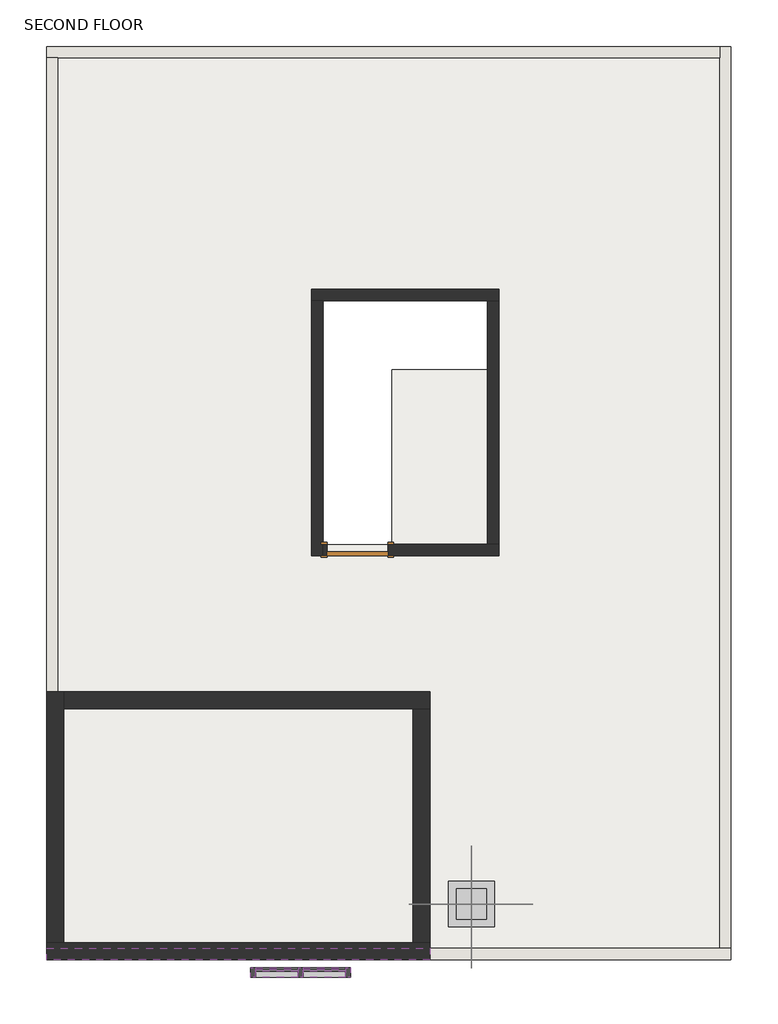
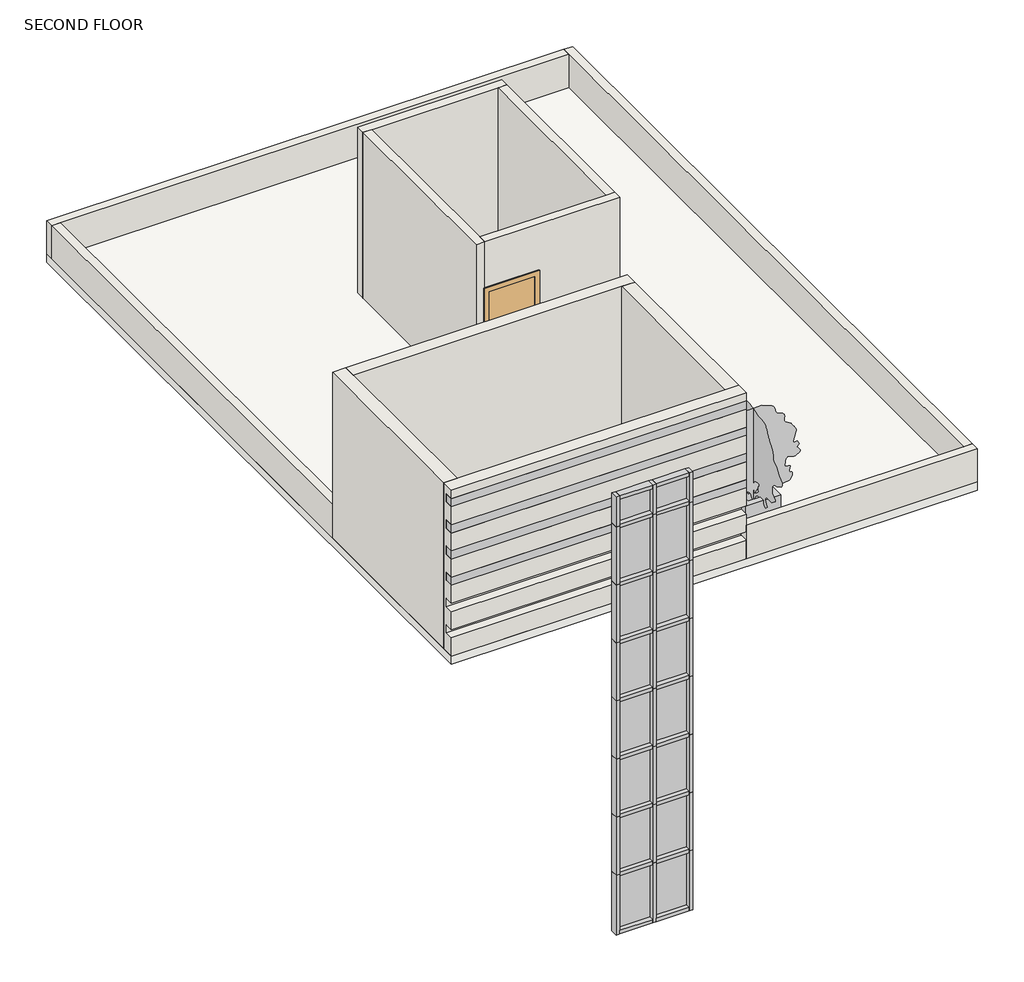
# One storey, incomplete: 42 members, 16 plates, 12 walls, 4 proxies, 2 geographic elements, 1 door, 1 slab.
"""IFC4 building model written with IfcOpenShell, lengths in millimetres."""

from ifc_helpers import new_model, si_unit, frame, origin, place, context, project, spatial, polyline, outline, extrude, faceted_brep, transform, mapped, element, save
from components import door_377e7377, planter_2_x2_da431093, rpc_tree_deciduous_largetooth_aspen_25_807f66b4, member_e80433b6, member_69c8e218, member_c8189573, member_de12db52, member_a715cb85, member_3683b620, member_544ec0ca, member_c4de40ee, system_panel_glazed_b36dd56d, system_panel_glazed_61a83ab7

model = new_model("IFC4")

# Units and contexts
model_context = context("Model", 3, world=origin())
ifc_project = project(units=[si_unit("LENGTHUNIT", "METRE", prefix="MILLI")], contexts=[model_context])

# Site, building, storey
site = spatial("IfcSite", under=ifc_project)
building = spatial("IfcBuilding", under=site)
storey = spatial("IfcBuildingStorey", under=building, Name="SECOND FLOOR", Elevation=6400.8)

# Proxies
placement = place(None, origin())
element("IfcBuildingElementProxy", 1, Name="Reveal", ObjectType="Reveal", at=placement, inside=storey, context=model_context, shape_type="SweptSolid", body=[
    extrude(outline(polyline([(-5827.2415084, -5557.8064015), (-5827.2415084, -5405.4064015), (-702.7915084, -5405.4064015), (-702.7915084, -5557.8064015), (-5827.2415084, -5557.8064015)])), frame((0.0, 0.0, 9144.0), z_axis=(0.0, 0.0, 1.0), x_axis=(1.0, 0.0, 0.0)), (0.0, 0.0, 1.0), 152.4),
])
element("IfcBuildingElementProxy", 2, Name="Reveal", ObjectType="Reveal", at=placement, inside=storey, context=model_context, shape_type="SweptSolid", body=[
    extrude(outline(polyline([(-5827.2415084, -5557.8064015), (-5827.2415084, -5405.4064015), (-702.7915084, -5405.4064015), (-702.7915084, -5557.8064015), (-5827.2415084, -5557.8064015)])), frame((0.0, 0.0, 8662.7368421), z_axis=(0.0, 0.0, 1.0), x_axis=(1.0, 0.0, 0.0)), (0.0, 0.0, 1.0), 152.4),
])
element("IfcBuildingElementProxy", 3, Name="Reveal", ObjectType="Reveal", at=placement, inside=storey, context=model_context, shape_type="SweptSolid", body=[
    extrude(outline(polyline([(-5827.2415084, -5557.8064015), (-5827.2415084, -5405.4064015), (-702.7915084, -5405.4064015), (-702.7915084, -5557.8064015), (-5827.2415084, -5557.8064015)])), frame((0.0, 0.0, 8181.4736842), z_axis=(0.0, 0.0, 1.0), x_axis=(1.0, 0.0, 0.0)), (0.0, 0.0, 1.0), 152.4),
])
element("IfcBuildingElementProxy", 4, Name="Reveal", ObjectType="Reveal", at=placement, inside=storey, context=model_context, shape_type="SweptSolid", body=[
    extrude(outline(polyline([(-5827.2415084, -5557.8064015), (-5827.2415084, -5405.4064015), (-702.7915084, -5405.4064015), (-702.7915084, -5557.8064015), (-5827.2415084, -5557.8064015)])), frame((0.0, 0.0, 7700.2105263), z_axis=(0.0, 0.0, 1.0), x_axis=(1.0, 0.0, 0.0)), (0.0, 0.0, 1.0), 152.4),
])

# Door
door_shape = door_377e7377(model_context)
element("IfcDoor", 5, ObjectType="Single-Flush : 2'8\"X7'", at=placement, inside=storey, context=model_context, shape_type="MappedRepresentation", body=[
    mapped(door_shape, transform((-1674.3415084, -85.6533727, 6400.8), x_axis=(-1.0, 0.0, 0.0), y_axis=(0.0, -1.0, 0.0), z_axis=(0.0, 0.0, 1.0))),
])

# Geographic elements
planter_2_x2_shape = planter_2_x2_da431093(model_context)
element("IfcGeographicElement", 6, ObjectType="Planter : 2'x2'", at=placement, inside=storey, context=model_context, shape_type="MappedRepresentation", body=[
    mapped(planter_2_x2_shape, transform((-150.3415084, -4814.8564015, 6400.8), x_axis=(1.0, 0.0, 0.0), y_axis=(0.0, 1.0, 0.0), z_axis=(0.0, 0.0, 1.0))),
])
rpc_tree_deciduous_largetooth_aspen_25_shape = rpc_tree_deciduous_largetooth_aspen_25_807f66b4(model_context)
element("IfcGeographicElement", 7, ObjectType="RPC Tree - Deciduous : Largetooth Aspen - 25'", at=placement, inside=storey, context=model_context, shape_type="MappedRepresentation", body=[
    mapped(rpc_tree_deciduous_largetooth_aspen_25_shape, transform((-150.3415084, -4814.8564015, 6400.8), x_axis=(1.0, 0.0, 0.0), y_axis=(0.0, 1.0, 0.0), z_axis=(0.0, 0.0, 1.0))),
])

# Members
member_shape = member_e80433b6(model_context)
element("IfcMember", 8, ObjectType="Rectangular Mullion : 2.5\" x 5\" rectangular", at=placement, inside=storey, context=model_context, shape_type="MappedRepresentation", body=[
    mapped(member_shape, transform((-2433.3720223, -5729.2564015, 462.2131579), x_axis=(1.0, 0.0, 0.0), y_axis=(0.0, -1.0, 0.0), z_axis=(0.0, 0.0, -1.0))),
])
member_2_shape = member_69c8e218(model_context)
element("IfcMember", 9, ObjectType="Rectangular Mullion : 2.5\" x 5\" rectangular", at=placement, inside=storey, context=model_context, shape_type="MappedRepresentation", body=[
    mapped(member_2_shape, transform((-1766.6220223, -5729.2564015, 462.2131579), x_axis=(1.0, 0.0, 0.0), y_axis=(0.0, -1.0, 0.0), z_axis=(0.0, 0.0, -1.0))),
])
member_3_shape = member_c8189573(model_context)
element("IfcMember", 10, ObjectType="Rectangular Mullion : 2.5\" x 5\" rectangular", at=placement, inside=storey, context=model_context, shape_type="MappedRepresentation", body=[
    mapped(member_3_shape, transform((-1830.1220223, -5729.2564015, 8510.3368421), x_axis=(0.0, 0.0, 1.0), y_axis=(0.0, -1.0, 0.0), z_axis=(1.0, 0.0, 0.0))),
])
element("IfcMember", 11, ObjectType="Rectangular Mullion : 2.5\" x 5\" rectangular", at=placement, inside=storey, context=model_context, shape_type="MappedRepresentation", body=[
    mapped(member_3_shape, transform((-2465.1220223, -5729.2564015, 8510.3368421), x_axis=(0.0, 0.0, 1.0), y_axis=(0.0, -1.0, 0.0), z_axis=(1.0, 0.0, 0.0))),
])
element("IfcMember", 12, ObjectType="Rectangular Mullion : 2.5\" x 5\" rectangular", at=placement, inside=storey, context=model_context, shape_type="MappedRepresentation", body=[
    mapped(member_3_shape, transform((-3036.6220223, -5729.2564015, 462.2131579), x_axis=(0.0, 0.0, -1.0), y_axis=(0.0, -1.0, 0.0), z_axis=(-1.0, 0.0, 0.0))),
])
element("IfcMember", 13, ObjectType="Rectangular Mullion : 2.5\" x 5\" rectangular", at=placement, inside=storey, context=model_context, shape_type="MappedRepresentation", body=[
    mapped(member_3_shape, transform((-2401.6220223, -5729.2564015, 462.2131579), x_axis=(0.0, 0.0, -1.0), y_axis=(0.0, -1.0, 0.0), z_axis=(-1.0, 0.0, 0.0))),
])
member_4_shape = member_de12db52(model_context)
element("IfcMember", 14, ObjectType="Rectangular Mullion : 2.5\" x 5\" rectangular", at=placement, inside=storey, context=model_context, shape_type="MappedRepresentation", body=[
    mapped(member_4_shape, transform((-2465.1220223, -5729.2564015, 1560.7631579), x_axis=(0.0, 0.0, 1.0), y_axis=(0.0, -1.0, 0.0), z_axis=(1.0, 0.0, 0.0))),
])
element("IfcMember", 15, ObjectType="Rectangular Mullion : 2.5\" x 5\" rectangular", at=placement, inside=storey, context=model_context, shape_type="MappedRepresentation", body=[
    mapped(member_4_shape, transform((-2465.1220223, -5729.2564015, 2627.5631579), x_axis=(0.0, 0.0, 1.0), y_axis=(0.0, -1.0, 0.0), z_axis=(1.0, 0.0, 0.0))),
])
element("IfcMember", 16, ObjectType="Rectangular Mullion : 2.5\" x 5\" rectangular", at=placement, inside=storey, context=model_context, shape_type="MappedRepresentation", body=[
    mapped(member_4_shape, transform((-2465.1220223, -5729.2564015, 3694.3631579), x_axis=(0.0, 0.0, 1.0), y_axis=(0.0, -1.0, 0.0), z_axis=(1.0, 0.0, 0.0))),
])
element("IfcMember", 17, ObjectType="Rectangular Mullion : 2.5\" x 5\" rectangular", at=placement, inside=storey, context=model_context, shape_type="MappedRepresentation", body=[
    mapped(member_4_shape, transform((-1830.1220223, -5729.2564015, 1560.7631579), x_axis=(0.0, 0.0, 1.0), y_axis=(0.0, -1.0, 0.0), z_axis=(1.0, 0.0, 0.0))),
])
element("IfcMember", 18, ObjectType="Rectangular Mullion : 2.5\" x 5\" rectangular", at=placement, inside=storey, context=model_context, shape_type="MappedRepresentation", body=[
    mapped(member_4_shape, transform((-1830.1220223, -5729.2564015, 2627.5631579), x_axis=(0.0, 0.0, 1.0), y_axis=(0.0, -1.0, 0.0), z_axis=(1.0, 0.0, 0.0))),
])
element("IfcMember", 19, ObjectType="Rectangular Mullion : 2.5\" x 5\" rectangular", at=placement, inside=storey, context=model_context, shape_type="MappedRepresentation", body=[
    mapped(member_4_shape, transform((-1830.1220223, -5729.2564015, 3694.3631579), x_axis=(0.0, 0.0, 1.0), y_axis=(0.0, -1.0, 0.0), z_axis=(1.0, 0.0, 0.0))),
])
element("IfcMember", 20, ObjectType="Rectangular Mullion : 2.5\" x 5\" rectangular", at=placement, inside=storey, context=model_context, shape_type="MappedRepresentation", body=[
    mapped(member_4_shape, transform((-2465.1220223, -5729.2564015, 4761.1631579), x_axis=(0.0, 0.0, 1.0), y_axis=(0.0, -1.0, 0.0), z_axis=(1.0, 0.0, 0.0))),
])
element("IfcMember", 21, ObjectType="Rectangular Mullion : 2.5\" x 5\" rectangular", at=placement, inside=storey, context=model_context, shape_type="MappedRepresentation", body=[
    mapped(member_4_shape, transform((-1830.1220223, -5729.2564015, 4761.1631579), x_axis=(0.0, 0.0, 1.0), y_axis=(0.0, -1.0, 0.0), z_axis=(1.0, 0.0, 0.0))),
])
element("IfcMember", 22, ObjectType="Rectangular Mullion : 2.5\" x 5\" rectangular", at=placement, inside=storey, context=model_context, shape_type="MappedRepresentation", body=[
    mapped(member_4_shape, transform((-2465.1220223, -5729.2564015, 5827.9631579), x_axis=(0.0, 0.0, 1.0), y_axis=(0.0, -1.0, 0.0), z_axis=(1.0, 0.0, 0.0))),
])
element("IfcMember", 23, ObjectType="Rectangular Mullion : 2.5\" x 5\" rectangular", at=placement, inside=storey, context=model_context, shape_type="MappedRepresentation", body=[
    mapped(member_4_shape, transform((-1830.1220223, -5729.2564015, 5827.9631579), x_axis=(0.0, 0.0, 1.0), y_axis=(0.0, -1.0, 0.0), z_axis=(1.0, 0.0, 0.0))),
])
element("IfcMember", 24, ObjectType="Rectangular Mullion : 2.5\" x 5\" rectangular", at=placement, inside=storey, context=model_context, shape_type="MappedRepresentation", body=[
    mapped(member_4_shape, transform((-2465.1220223, -5729.2564015, 6894.7631579), x_axis=(0.0, 0.0, 1.0), y_axis=(0.0, -1.0, 0.0), z_axis=(1.0, 0.0, 0.0))),
])
element("IfcMember", 25, ObjectType="Rectangular Mullion : 2.5\" x 5\" rectangular", at=placement, inside=storey, context=model_context, shape_type="MappedRepresentation", body=[
    mapped(member_4_shape, transform((-1830.1220223, -5729.2564015, 6894.7631579), x_axis=(0.0, 0.0, 1.0), y_axis=(0.0, -1.0, 0.0), z_axis=(1.0, 0.0, 0.0))),
])
element("IfcMember", 26, ObjectType="Rectangular Mullion : 2.5\" x 5\" rectangular", at=placement, inside=storey, context=model_context, shape_type="MappedRepresentation", body=[
    mapped(member_4_shape, transform((-2465.1220223, -5729.2564015, 7961.5631579), x_axis=(0.0, 0.0, 1.0), y_axis=(0.0, -1.0, 0.0), z_axis=(1.0, 0.0, 0.0))),
])
element("IfcMember", 27, ObjectType="Rectangular Mullion : 2.5\" x 5\" rectangular", at=placement, inside=storey, context=model_context, shape_type="MappedRepresentation", body=[
    mapped(member_4_shape, transform((-1830.1220223, -5729.2564015, 7961.5631579), x_axis=(0.0, 0.0, 1.0), y_axis=(0.0, -1.0, 0.0), z_axis=(1.0, 0.0, 0.0))),
])
member_5_shape = member_a715cb85(model_context)
element("IfcMember", 28, ObjectType="Rectangular Mullion : 2.5\" x 5\" rectangular", at=placement, inside=storey, context=model_context, shape_type="MappedRepresentation", body=[
    mapped(member_5_shape, transform((-2433.3720223, -5729.2564015, 1560.7631579), x_axis=(1.0, 0.0, 0.0), y_axis=(0.0, -1.0, 0.0), z_axis=(0.0, 0.0, -1.0))),
])
element("IfcMember", 29, ObjectType="Rectangular Mullion : 2.5\" x 5\" rectangular", at=placement, inside=storey, context=model_context, shape_type="MappedRepresentation", body=[
    mapped(member_5_shape, transform((-2433.3720223, -5729.2564015, 2627.5631579), x_axis=(1.0, 0.0, 0.0), y_axis=(0.0, -1.0, 0.0), z_axis=(0.0, 0.0, -1.0))),
])
element("IfcMember", 30, ObjectType="Rectangular Mullion : 2.5\" x 5\" rectangular", at=placement, inside=storey, context=model_context, shape_type="MappedRepresentation", body=[
    mapped(member_5_shape, transform((-2433.3720223, -5729.2564015, 3694.3631579), x_axis=(1.0, 0.0, 0.0), y_axis=(0.0, -1.0, 0.0), z_axis=(0.0, 0.0, -1.0))),
])
element("IfcMember", 31, ObjectType="Rectangular Mullion : 2.5\" x 5\" rectangular", at=placement, inside=storey, context=model_context, shape_type="MappedRepresentation", body=[
    mapped(member_5_shape, transform((-2433.3720223, -5729.2564015, 4761.1631579), x_axis=(1.0, 0.0, 0.0), y_axis=(0.0, -1.0, 0.0), z_axis=(0.0, 0.0, -1.0))),
])
element("IfcMember", 32, ObjectType="Rectangular Mullion : 2.5\" x 5\" rectangular", at=placement, inside=storey, context=model_context, shape_type="MappedRepresentation", body=[
    mapped(member_5_shape, transform((-2433.3720223, -5729.2564015, 5827.9631579), x_axis=(1.0, 0.0, 0.0), y_axis=(0.0, -1.0, 0.0), z_axis=(0.0, 0.0, -1.0))),
])
element("IfcMember", 33, ObjectType="Rectangular Mullion : 2.5\" x 5\" rectangular", at=placement, inside=storey, context=model_context, shape_type="MappedRepresentation", body=[
    mapped(member_5_shape, transform((-2433.3720223, -5729.2564015, 6894.7631579), x_axis=(1.0, 0.0, 0.0), y_axis=(0.0, -1.0, 0.0), z_axis=(0.0, 0.0, -1.0))),
])
member_6_shape = member_3683b620(model_context)
element("IfcMember", 34, ObjectType="Rectangular Mullion : 2.5\" x 5\" rectangular", at=placement, inside=storey, context=model_context, shape_type="MappedRepresentation", body=[
    mapped(member_6_shape, transform((-2433.3720223, -5729.2564015, 7961.5631579), x_axis=(1.0, 0.0, 0.0), y_axis=(0.0, -1.0, 0.0), z_axis=(0.0, 0.0, -1.0))),
])
member_7_shape = member_544ec0ca(model_context)
element("IfcMember", 35, ObjectType="Rectangular Mullion : 2.5\" x 5\" rectangular", at=placement, inside=storey, context=model_context, shape_type="MappedRepresentation", body=[
    mapped(member_7_shape, transform((-3100.1220223, -5729.2564015, 8510.3368421), x_axis=(-1.0, 0.0, 0.0), y_axis=(0.0, -1.0, 0.0), z_axis=(0.0, 0.0, 1.0))),
])
member_8_shape = member_c4de40ee(model_context)
element("IfcMember", 36, ObjectType="Rectangular Mullion : 2.5\" x 5\" rectangular", at=placement, inside=storey, context=model_context, shape_type="MappedRepresentation", body=[
    mapped(member_8_shape, transform((-1766.6220223, -5729.2564015, 1560.7631579), x_axis=(1.0, 0.0, 0.0), y_axis=(0.0, -1.0, 0.0), z_axis=(0.0, 0.0, -1.0))),
])
element("IfcMember", 37, ObjectType="Rectangular Mullion : 2.5\" x 5\" rectangular", at=placement, inside=storey, context=model_context, shape_type="MappedRepresentation", body=[
    mapped(member_8_shape, transform((-1766.6220223, -5729.2564015, 2627.5631579), x_axis=(1.0, 0.0, 0.0), y_axis=(0.0, -1.0, 0.0), z_axis=(0.0, 0.0, -1.0))),
])
element("IfcMember", 38, ObjectType="Rectangular Mullion : 2.5\" x 5\" rectangular", at=placement, inside=storey, context=model_context, shape_type="MappedRepresentation", body=[
    mapped(member_8_shape, transform((-1766.6220223, -5729.2564015, 3694.3631579), x_axis=(1.0, 0.0, 0.0), y_axis=(0.0, -1.0, 0.0), z_axis=(0.0, 0.0, -1.0))),
])
element("IfcMember", 39, ObjectType="Rectangular Mullion : 2.5\" x 5\" rectangular", at=placement, inside=storey, context=model_context, shape_type="MappedRepresentation", body=[
    mapped(member_8_shape, transform((-1766.6220223, -5729.2564015, 4761.1631579), x_axis=(1.0, 0.0, 0.0), y_axis=(0.0, -1.0, 0.0), z_axis=(0.0, 0.0, -1.0))),
])
element("IfcMember", 40, ObjectType="Rectangular Mullion : 2.5\" x 5\" rectangular", at=placement, inside=storey, context=model_context, shape_type="MappedRepresentation", body=[
    mapped(member_8_shape, transform((-1766.6220223, -5729.2564015, 5827.9631579), x_axis=(1.0, 0.0, 0.0), y_axis=(0.0, -1.0, 0.0), z_axis=(0.0, 0.0, -1.0))),
])
element("IfcMember", 41, ObjectType="Rectangular Mullion : 2.5\" x 5\" rectangular", at=placement, inside=storey, context=model_context, shape_type="MappedRepresentation", body=[
    mapped(member_8_shape, transform((-1766.6220223, -5729.2564015, 6894.7631579), x_axis=(1.0, 0.0, 0.0), y_axis=(0.0, -1.0, 0.0), z_axis=(0.0, 0.0, -1.0))),
])
element("IfcMember", 42, ObjectType="Rectangular Mullion : 2.5\" x 5\" rectangular", at=placement, inside=storey, context=model_context, shape_type="MappedRepresentation", body=[
    mapped(member_2_shape, transform((-3100.1220223, -5729.2564015, 1560.7631579), x_axis=(-1.0, 0.0, 0.0), y_axis=(0.0, -1.0, 0.0), z_axis=(0.0, 0.0, 1.0))),
])
element("IfcMember", 43, ObjectType="Rectangular Mullion : 2.5\" x 5\" rectangular", at=placement, inside=storey, context=model_context, shape_type="MappedRepresentation", body=[
    mapped(member_8_shape, transform((-3100.1220223, -5729.2564015, 2627.5631579), x_axis=(-1.0, 0.0, 0.0), y_axis=(0.0, -1.0, 0.0), z_axis=(0.0, 0.0, 1.0))),
])
element("IfcMember", 44, ObjectType="Rectangular Mullion : 2.5\" x 5\" rectangular", at=placement, inside=storey, context=model_context, shape_type="MappedRepresentation", body=[
    mapped(member_8_shape, transform((-3100.1220223, -5729.2564015, 3694.3631579), x_axis=(-1.0, 0.0, 0.0), y_axis=(0.0, -1.0, 0.0), z_axis=(0.0, 0.0, 1.0))),
])
element("IfcMember", 45, ObjectType="Rectangular Mullion : 2.5\" x 5\" rectangular", at=placement, inside=storey, context=model_context, shape_type="MappedRepresentation", body=[
    mapped(member_8_shape, transform((-3100.1220223, -5729.2564015, 4761.1631579), x_axis=(-1.0, 0.0, 0.0), y_axis=(0.0, -1.0, 0.0), z_axis=(0.0, 0.0, 1.0))),
])
element("IfcMember", 46, ObjectType="Rectangular Mullion : 2.5\" x 5\" rectangular", at=placement, inside=storey, context=model_context, shape_type="MappedRepresentation", body=[
    mapped(member_8_shape, transform((-3100.1220223, -5729.2564015, 5827.9631579), x_axis=(-1.0, 0.0, 0.0), y_axis=(0.0, -1.0, 0.0), z_axis=(0.0, 0.0, 1.0))),
])
element("IfcMember", 47, ObjectType="Rectangular Mullion : 2.5\" x 5\" rectangular", at=placement, inside=storey, context=model_context, shape_type="MappedRepresentation", body=[
    mapped(member_8_shape, transform((-3100.1220223, -5729.2564015, 6894.7631579), x_axis=(-1.0, 0.0, 0.0), y_axis=(0.0, -1.0, 0.0), z_axis=(0.0, 0.0, 1.0))),
])
element("IfcMember", 48, ObjectType="Rectangular Mullion : 2.5\" x 5\" rectangular", at=placement, inside=storey, context=model_context, shape_type="MappedRepresentation", body=[
    mapped(member_8_shape, transform((-3100.1220223, -5729.2564015, 7961.5631579), x_axis=(-1.0, 0.0, 0.0), y_axis=(0.0, -1.0, 0.0), z_axis=(0.0, 0.0, 1.0))),
])
element("IfcMember", 49, ObjectType="Rectangular Mullion : 2.5\" x 5\" rectangular", at=placement, inside=storey, context=model_context, shape_type="MappedRepresentation", body=[
    mapped(member_7_shape, transform((-1766.6220223, -5729.2564015, 7961.5631579), x_axis=(1.0, 0.0, 0.0), y_axis=(0.0, -1.0, 0.0), z_axis=(0.0, 0.0, -1.0))),
])

# Plates
system_panel_glazed_shape = system_panel_glazed_b36dd56d(model_context)
element("IfcPlate", 50, ObjectType="System Panel : Glazed", at=placement, inside=storey, context=model_context, shape_type="MappedRepresentation", body=[
    mapped(system_panel_glazed_shape, transform((-2750.8720223, -5729.2564015, 525.7131579), x_axis=(1.0, 0.0, 0.0), y_axis=(0.0, 1.0, 0.0), z_axis=(0.0, 0.0, 1.0))),
])
element("IfcPlate", 51, ObjectType="System Panel : Glazed", at=placement, inside=storey, context=model_context, shape_type="MappedRepresentation", body=[
    mapped(system_panel_glazed_shape, transform((-2750.8720223, -5729.2564015, 1592.5131579), x_axis=(1.0, 0.0, 0.0), y_axis=(0.0, 1.0, 0.0), z_axis=(0.0, 0.0, 1.0))),
])
element("IfcPlate", 52, ObjectType="System Panel : Glazed", at=placement, inside=storey, context=model_context, shape_type="MappedRepresentation", body=[
    mapped(system_panel_glazed_shape, transform((-2750.8720223, -5729.2564015, 2659.3131579), x_axis=(1.0, 0.0, 0.0), y_axis=(0.0, 1.0, 0.0), z_axis=(0.0, 0.0, 1.0))),
])
element("IfcPlate", 53, ObjectType="System Panel : Glazed", at=placement, inside=storey, context=model_context, shape_type="MappedRepresentation", body=[
    mapped(system_panel_glazed_shape, transform((-2750.8720223, -5729.2564015, 3726.1131579), x_axis=(1.0, 0.0, 0.0), y_axis=(0.0, 1.0, 0.0), z_axis=(0.0, 0.0, 1.0))),
])
element("IfcPlate", 54, ObjectType="System Panel : Glazed", at=placement, inside=storey, context=model_context, shape_type="MappedRepresentation", body=[
    mapped(system_panel_glazed_shape, transform((-2115.8720223, -5729.2564015, 525.7131579), x_axis=(1.0, 0.0, 0.0), y_axis=(0.0, 1.0, 0.0), z_axis=(0.0, 0.0, 1.0))),
])
element("IfcPlate", 55, ObjectType="System Panel : Glazed", at=placement, inside=storey, context=model_context, shape_type="MappedRepresentation", body=[
    mapped(system_panel_glazed_shape, transform((-2115.8720223, -5729.2564015, 1592.5131579), x_axis=(1.0, 0.0, 0.0), y_axis=(0.0, 1.0, 0.0), z_axis=(0.0, 0.0, 1.0))),
])
element("IfcPlate", 56, ObjectType="System Panel : Glazed", at=placement, inside=storey, context=model_context, shape_type="MappedRepresentation", body=[
    mapped(system_panel_glazed_shape, transform((-2115.8720223, -5729.2564015, 2659.3131579), x_axis=(1.0, 0.0, 0.0), y_axis=(0.0, 1.0, 0.0), z_axis=(0.0, 0.0, 1.0))),
])
element("IfcPlate", 57, ObjectType="System Panel : Glazed", at=placement, inside=storey, context=model_context, shape_type="MappedRepresentation", body=[
    mapped(system_panel_glazed_shape, transform((-2115.8720223, -5729.2564015, 3726.1131579), x_axis=(1.0, 0.0, 0.0), y_axis=(0.0, 1.0, 0.0), z_axis=(0.0, 0.0, 1.0))),
])
element("IfcPlate", 58, ObjectType="System Panel : Glazed", at=placement, inside=storey, context=model_context, shape_type="MappedRepresentation", body=[
    mapped(system_panel_glazed_shape, transform((-2750.8720223, -5729.2564015, 4792.9131579), x_axis=(1.0, 0.0, 0.0), y_axis=(0.0, 1.0, 0.0), z_axis=(0.0, 0.0, 1.0))),
])
element("IfcPlate", 59, ObjectType="System Panel : Glazed", at=placement, inside=storey, context=model_context, shape_type="MappedRepresentation", body=[
    mapped(system_panel_glazed_shape, transform((-2115.8720223, -5729.2564015, 4792.9131579), x_axis=(1.0, 0.0, 0.0), y_axis=(0.0, 1.0, 0.0), z_axis=(0.0, 0.0, 1.0))),
])
element("IfcPlate", 60, ObjectType="System Panel : Glazed", at=placement, inside=storey, context=model_context, shape_type="MappedRepresentation", body=[
    mapped(system_panel_glazed_shape, transform((-2750.8720223, -5729.2564015, 5859.7131579), x_axis=(1.0, 0.0, 0.0), y_axis=(0.0, 1.0, 0.0), z_axis=(0.0, 0.0, 1.0))),
])
element("IfcPlate", 61, ObjectType="System Panel : Glazed", at=placement, inside=storey, context=model_context, shape_type="MappedRepresentation", body=[
    mapped(system_panel_glazed_shape, transform((-2115.8720223, -5729.2564015, 5859.7131579), x_axis=(1.0, 0.0, 0.0), y_axis=(0.0, 1.0, 0.0), z_axis=(0.0, 0.0, 1.0))),
])
element("IfcPlate", 62, ObjectType="System Panel : Glazed", at=placement, inside=storey, context=model_context, shape_type="MappedRepresentation", body=[
    mapped(system_panel_glazed_shape, transform((-2750.8720223, -5729.2564015, 6926.5131579), x_axis=(1.0, 0.0, 0.0), y_axis=(0.0, 1.0, 0.0), z_axis=(0.0, 0.0, 1.0))),
])
element("IfcPlate", 63, ObjectType="System Panel : Glazed", at=placement, inside=storey, context=model_context, shape_type="MappedRepresentation", body=[
    mapped(system_panel_glazed_shape, transform((-2115.8720223, -5729.2564015, 6926.5131579), x_axis=(1.0, 0.0, 0.0), y_axis=(0.0, 1.0, 0.0), z_axis=(0.0, 0.0, 1.0))),
])
system_panel_glazed_2_shape = system_panel_glazed_61a83ab7(model_context)
element("IfcPlate", 64, ObjectType="System Panel : Glazed", at=placement, inside=storey, context=model_context, shape_type="MappedRepresentation", body=[
    mapped(system_panel_glazed_2_shape, transform((-2750.8720223, -5729.2564015, 7993.3131579), x_axis=(1.0, 0.0, 0.0), y_axis=(0.0, 1.0, 0.0), z_axis=(0.0, 0.0, 1.0))),
])
element("IfcPlate", 65, ObjectType="System Panel : Glazed", at=placement, inside=storey, context=model_context, shape_type="MappedRepresentation", body=[
    mapped(system_panel_glazed_2_shape, transform((-2115.8720223, -5729.2564015, 7993.3131579), x_axis=(1.0, 0.0, 0.0), y_axis=(0.0, 1.0, 0.0), z_axis=(0.0, 0.0, 1.0))),
])

# Slab
element("IfcSlab", 66, ObjectType="6\"", at=placement, inside=storey, context=model_context, shape_type="SweptSolid", body=[
    extrude(outline(polyline([(3316.7584916, 6634.1935985), (3316.7584916, -5557.8064015), (-5827.2415084, -5557.8064015), (-5827.2415084, 6634.1935985), (3316.7584916, 6634.1935985)]), holes=[polyline([(-2131.5415084, 3243.2935985), (-2131.5415084, -9.4533727), (-1217.1415084, -9.4533727), (-1217.1415084, 2328.8935985), (65.5584916, 2328.8935985), (65.5584916, 3243.2935985), (-2131.5415084, 3243.2935985)])]), frame((0.0, 0.0, 6248.4), z_axis=(0.0, 0.0, 1.0), x_axis=(1.0, 0.0, 0.0)), (0.0, 0.0, 1.0), 152.4),
])

# Walls
element("IfcWall", 67, ObjectType="6\"", at=placement, inside=storey, context=model_context, shape_type="Brep", body=[
    faceted_brep([(217.9584916, 3395.6935985, 6400.8), (-2283.9415084, 3395.6935985, 6400.8), (-2283.9415084, 3395.6935985, 9448.8), (217.9584916, 3395.6935985, 9448.8), (217.9584916, 3243.2935985, 6400.8), (217.9584916, 3243.2935985, 9448.8), (65.5584916, 3243.2935985, 9448.8), (-2131.5415084, 3243.2935985, 9448.8), (-2283.9415084, 3243.2935985, 9448.8), (-2283.9415084, 3243.2935985, 6400.8), (-2131.5415084, 3243.2935985, 6400.8), (65.5584916, 3243.2935985, 6400.8)], [[[0, 1, 2, 3]], [[4, 5, 6, 7, 8, 9, 10, 11]], [[1, 0, 4, 11, 10, 9]], [[3, 2, 8, 7, 6, 5]], [[2, 1, 9, 8]], [[0, 3, 5, 4]]]),
])
element("IfcWall", 68, ObjectType="6\"", at=placement, inside=storey, context=model_context, shape_type="Brep", body=[
    faceted_brep([(-2283.9415084, 3243.2935985, 6400.8), (-2283.9415084, -161.8533727, 6400.8), (-2283.9415084, -161.8533727, 9448.8), (-2283.9415084, 3243.2935985, 9448.8), (-2131.5415084, 3243.2935985, 6400.8), (-2131.5415084, 3243.2935985, 9448.8), (-2131.5415084, -9.4533727, 9448.8), (-2131.5415084, -161.8533727, 9448.8), (-2131.5415084, -161.8533727, 6400.8), (-2131.5415084, -9.4533727, 6400.8)], [[[0, 1, 2, 3]], [[4, 5, 6, 7, 8, 9]], [[1, 0, 4, 9, 8]], [[3, 2, 7, 6, 5]], [[0, 3, 5, 4]], [[2, 1, 8, 7]]]),
])
element("IfcWall", 69, ObjectType="6\"", at=placement, inside=storey, context=model_context, shape_type="Brep", body=[
    faceted_brep([(-2131.5415084, -161.8533727, 6400.8), (-2080.7415084, -161.8533727, 6400.8), (-2080.7415084, -161.8533727, 8534.4), (-1267.9415084, -161.8533727, 8534.4), (-1267.9415084, -161.8533727, 6400.8), (217.9584916, -161.8533727, 6400.8), (217.9584916, -161.8533727, 9448.8), (-2131.5415084, -161.8533727, 9448.8), (-2080.7415084, -9.4533727, 8534.4), (-2080.7415084, -9.4533727, 6400.8), (-2131.5415084, -9.4533727, 6400.8), (-2131.5415084, -9.4533727, 9448.8), (65.5584916, -9.4533727, 9448.8), (217.9584916, -9.4533727, 9448.8), (217.9584916, -9.4533727, 6400.8), (65.5584916, -9.4533727, 6400.8), (-1267.9415084, -9.4533727, 6400.8), (-1267.9415084, -9.4533727, 8534.4)], [[[0, 1, 2, 3, 4, 5, 6, 7]], [[8, 9, 10, 11, 12, 13, 14, 15, 16, 17]], [[10, 9, 1, 0]], [[16, 15, 14, 5, 4]], [[7, 6, 13, 12, 11]], [[0, 7, 11, 10]], [[6, 5, 14, 13]], [[2, 1, 9, 8]], [[3, 2, 8, 17]], [[4, 3, 17, 16]]]),
])
element("IfcWall", 70, ObjectType="6\"", at=placement, inside=storey, context=model_context, shape_type="SweptSolid", body=[
    extrude(outline(polyline([(217.9584916, 3243.2935985), (217.9584916, -9.4533727), (65.5584916, -9.4533727), (65.5584916, 3243.2935985), (217.9584916, 3243.2935985)])), frame((0.0, 0.0, 6400.8), z_axis=(0.0, 0.0, 1.0), x_axis=(1.0, 0.0, 0.0)), (0.0, 0.0, 1.0), 3048.0),
])
element("IfcWall", 71, ObjectType="6\"", at=placement, inside=storey, context=model_context, shape_type="Brep", body=[
    faceted_brep([(-702.7915084, -5557.8064015, 6400.8), (3316.7584916, -5557.8064015, 6400.8), (3316.7584916, -5557.8064015, 7010.4), (-702.7915084, -5557.8064015, 7010.4), (-702.7915084, -5557.8064015, 6890.0842105), (-702.7915084, -5557.8064015, 6737.6842105), (-702.7915084, -5405.4064015, 6400.8), (-702.7915084, -5405.4064015, 7010.4), (3164.3584916, -5405.4064015, 7010.4), (3316.7584916, -5405.4064015, 7010.4), (3316.7584916, -5405.4064015, 6400.8), (3164.3584916, -5405.4064015, 6400.8)], [[[0, 1, 2, 3, 4, 5]], [[6, 7, 8, 9, 10, 11]], [[1, 0, 6, 11, 10]], [[3, 2, 9, 8, 7]], [[0, 5, 4, 3, 7, 6]], [[2, 1, 10, 9]]]),
])
element("IfcWall", 72, ObjectType="6\"", at=placement, inside=storey, context=model_context, shape_type="Brep", body=[
    faceted_brep([(3316.7584916, -5405.4064015, 6400.8), (3316.7584916, 6634.1935985, 6400.8), (3316.7584916, 6634.1935985, 7010.4), (3316.7584916, -5405.4064015, 7010.4), (3164.3584916, -5405.4064015, 6400.8), (3164.3584916, -5405.4064015, 7010.4), (3164.3584916, 6481.7935985, 7010.4), (3164.3584916, 6634.1935985, 7010.4), (3164.3584916, 6634.1935985, 6400.8), (3164.3584916, 6481.7935985, 6400.8)], [[[0, 1, 2, 3]], [[4, 5, 6, 7, 8, 9]], [[1, 0, 4, 9, 8]], [[3, 2, 7, 6, 5]], [[0, 3, 5, 4]], [[2, 1, 8, 7]]]),
])
element("IfcWall", 73, ObjectType="6\"", at=placement, inside=storey, context=model_context, shape_type="Brep", body=[
    faceted_brep([(3164.3584916, 6634.1935985, 6400.8), (-5827.2415084, 6634.1935985, 6400.8), (-5827.2415084, 6634.1935985, 7010.4), (3164.3584916, 6634.1935985, 7010.4), (3164.3584916, 6481.7935985, 6400.8), (3164.3584916, 6481.7935985, 7010.4), (-5674.8415084, 6481.7935985, 7010.4), (-5827.2415084, 6481.7935985, 7010.4), (-5827.2415084, 6481.7935985, 6400.8), (-5674.8415084, 6481.7935985, 6400.8)], [[[0, 1, 2, 3]], [[4, 5, 6, 7, 8, 9]], [[1, 0, 4, 9, 8]], [[3, 2, 7, 6, 5]], [[0, 3, 5, 4]], [[2, 1, 8, 7]]]),
])
element("IfcWall", 74, ObjectType="6\"", at=placement, inside=storey, context=model_context, shape_type="SweptSolid", body=[
    extrude(outline(polyline([(-5827.2415084, -1976.4064015), (-5827.2415084, 6481.7935985), (-5674.8415084, 6481.7935985), (-5674.8415084, -1976.4064015), (-5827.2415084, -1976.4064015)])), frame((0.0, 0.0, 6400.8), z_axis=(0.0, 0.0, 1.0), x_axis=(1.0, 0.0, 0.0)), (0.0, 0.0, 1.0), 609.6),
])
element("IfcWall", 75, ObjectType="9\"", at=placement, inside=storey, context=model_context, shape_type="Brep", body=[
    faceted_brep([(-5827.2415084, -5557.8064015, 6400.8), (-702.7915084, -5557.8064015, 6400.8), (-702.7915084, -5557.8064015, 6737.6842105), (-5827.2415084, -5557.8064015, 6737.6842105), (-702.7915084, -5557.8064015, 9448.8), (-5827.2415084, -5557.8064015, 9448.8), (-5827.2415084, -5557.8064015, 9296.4), (-702.7915084, -5557.8064015, 9296.4), (-702.7915084, -5557.8064015, 9144.0), (-5827.2415084, -5557.8064015, 9144.0), (-5827.2415084, -5557.8064015, 8815.1368421), (-702.7915084, -5557.8064015, 8815.1368421), (-5827.2415084, -5557.8064015, 6890.0842105), (-702.7915084, -5557.8064015, 6890.0842105), (-702.7915084, -5557.8064015, 7218.9473684), (-5827.2415084, -5557.8064015, 7218.9473684), (-5827.2415084, -5557.8064015, 7371.3473684), (-702.7915084, -5557.8064015, 7371.3473684), (-702.7915084, -5557.8064015, 7700.2105263), (-5827.2415084, -5557.8064015, 7700.2105263), (-5827.2415084, -5557.8064015, 7852.6105263), (-702.7915084, -5557.8064015, 7852.6105263), (-702.7915084, -5557.8064015, 8181.4736842), (-5827.2415084, -5557.8064015, 8181.4736842), (-5827.2415084, -5557.8064015, 8333.8736842), (-702.7915084, -5557.8064015, 8333.8736842), (-702.7915084, -5557.8064015, 8662.7368421), (-5827.2415084, -5557.8064015, 8662.7368421), (-702.7915084, -5329.2064015, 6400.8), (-931.3915084, -5329.2064015, 6400.8), (-5598.6415084, -5329.2064015, 6400.8), (-5827.2415084, -5329.2064015, 6400.8), (-5827.2415084, -5329.2064015, 9448.8), (-5598.6415084, -5329.2064015, 9448.8), (-931.3915084, -5329.2064015, 9448.8), (-702.7915084, -5329.2064015, 9448.8), (-702.7915084, -5405.4064015, 6400.8), (-5827.2415084, -5405.4064015, 6737.6842105), (-5827.2415084, -5405.4064015, 6890.0842105), (-5827.2415084, -5405.4064015, 7218.9473684), (-5827.2415084, -5405.4064015, 7371.3473684), (-5827.2415084, -5405.4064015, 7700.2105263), (-5827.2415084, -5405.4064015, 7852.6105263), (-5827.2415084, -5405.4064015, 8181.4736842), (-5827.2415084, -5405.4064015, 8333.8736842), (-5827.2415084, -5405.4064015, 8662.7368421), (-5827.2415084, -5405.4064015, 8815.1368421), (-5827.2415084, -5405.4064015, 9144.0), (-5827.2415084, -5405.4064015, 9296.4), (-702.7915084, -5405.4064015, 9296.4), (-702.7915084, -5405.4064015, 9144.0), (-702.7915084, -5405.4064015, 6890.0842105), (-702.7915084, -5405.4064015, 6737.6842105), (-702.7915084, -5405.4064015, 7371.3473684), (-702.7915084, -5405.4064015, 7218.9473684), (-702.7915084, -5405.4064015, 7852.6105263), (-702.7915084, -5405.4064015, 7700.2105263), (-702.7915084, -5405.4064015, 8333.8736842), (-702.7915084, -5405.4064015, 8181.4736842), (-702.7915084, -5405.4064015, 8815.1368421), (-702.7915084, -5405.4064015, 8662.7368421)], [[[0, 1, 2, 3]], [[4, 5, 6, 7]], [[8, 9, 10, 11]], [[12, 13, 14, 15]], [[16, 17, 18, 19]], [[20, 21, 22, 23]], [[24, 25, 26, 27]], [[28, 29, 30, 31, 32, 33, 34, 35]], [[1, 0, 31, 30, 29, 28, 36]], [[5, 4, 35, 34, 33, 32]], [[5, 32, 31, 0, 3, 37, 38, 12, 15, 39, 40, 16, 19, 41, 42, 20, 23, 43, 44, 24, 27, 45, 46, 10, 9, 47, 48, 6]], [[48, 49, 7, 6]], [[49, 48, 47, 50]], [[50, 47, 9, 8]], [[38, 51, 13, 12]], [[51, 38, 37, 52]], [[52, 37, 3, 2]], [[40, 53, 17, 16]], [[53, 40, 39, 54]], [[54, 39, 15, 14]], [[42, 55, 21, 20]], [[55, 42, 41, 56]], [[56, 41, 19, 18]], [[44, 57, 25, 24]], [[57, 44, 43, 58]], [[58, 43, 23, 22]], [[46, 59, 11, 10]], [[59, 46, 45, 60]], [[60, 45, 27, 26]], [[1, 36, 28, 35, 4, 7, 49, 50, 8, 11, 59, 60, 26, 25, 57, 58, 22, 21, 55, 56, 18, 17, 53, 54, 14, 13, 51, 52, 2]]]),
])
element("IfcWall", 76, ObjectType="9\"", at=placement, inside=storey, context=model_context, shape_type="Brep", body=[
    faceted_brep([(-5598.6415084, -5329.2064015, 6400.8), (-5598.6415084, -2205.0064015, 6400.8), (-5598.6415084, -1976.4064015, 6400.8), (-5598.6415084, -1976.4064015, 9448.8), (-5598.6415084, -2205.0064015, 9448.8), (-5598.6415084, -5329.2064015, 9448.8), (-5827.2415084, -5329.2064015, 6400.8), (-5827.2415084, -5329.2064015, 9448.8), (-5827.2415084, -1976.4064015, 9448.8), (-5827.2415084, -1976.4064015, 7010.4), (-5827.2415084, -1976.4064015, 6400.8), (-5674.8415084, -1976.4064015, 6400.8)], [[[0, 1, 2, 3, 4, 5]], [[6, 7, 8, 9, 10]], [[2, 1, 0, 6, 10, 11]], [[5, 4, 3, 8, 7]], [[0, 5, 7, 6]], [[2, 11, 10, 9, 8, 3]]]),
])
element("IfcWall", 77, ObjectType="9\"", at=placement, inside=storey, context=model_context, shape_type="Brep", body=[
    faceted_brep([(-5598.6415084, -2205.0064015, 9448.8), (-5598.6415084, -2205.0064015, 6400.8), (-931.3915084, -2205.0064015, 6400.8), (-702.7915084, -2205.0064015, 6400.8), (-702.7915084, -2205.0064015, 9448.8), (-931.3915084, -2205.0064015, 9448.8), (-5598.6415084, -1976.4064015, 6400.8), (-5598.6415084, -1976.4064015, 9448.8), (-702.7915084, -1976.4064015, 9448.8), (-702.7915084, -1976.4064015, 6400.8)], [[[0, 1, 2, 3, 4, 5]], [[6, 7, 8, 9]], [[3, 2, 1, 6, 9]], [[0, 5, 4, 8, 7]], [[4, 3, 9, 8]], [[0, 7, 6, 1]]]),
])
element("IfcWall", 78, ObjectType="9\"", at=placement, inside=storey, context=model_context, shape_type="SweptSolid", body=[
    extrude(outline(polyline([(-931.3915084, -5329.2064015), (-931.3915084, -2205.0064015), (-702.7915084, -2205.0064015), (-702.7915084, -5329.2064015), (-931.3915084, -5329.2064015)])), frame((0.0, 0.0, 6400.8), z_axis=(0.0, 0.0, 1.0), x_axis=(1.0, 0.0, 0.0)), (0.0, 0.0, 1.0), 3048.0),
])

save(model, "model.ifc")

# Revit data of these elements
# Type "Single-Flush : 2'8\"X7'"
#   Type Mark = "9"
#   Construction Type Id = "MDOOR"
#   Assembly Code = "C1020"
#   Analytic Construction = "Metal"
#   Thickness = 0' - 2"
#   Heat Transfer Coefficient (U) = 0.651978 BTU/(h·ft²·°F)
#   Height = 7' - 0"
#   Trim Projection Ext = 0' - 1"
#   Trim Projection Int = 0' - 1"
#   Trim Width = 0' - 3"
#   Width = 2' - 8"
#   Define Thermal Properties by = 1
#   Door Material = Door - Panel
#   Frame Material = Door - Frame
#   Visual Light Transmittance = 0
#   Solar Heat Gain Coefficient = 0
#   Function = (empty or 0)
#   Wall Closure = (empty or 0)
# Type "Planter : 2'x2'"
#   Depth = 2' - 0"
#   Height = 2' - 0"
#   Width = 2' - 0"
#   Material = Concrete, Precast
# Type "RPC Tree - Deciduous : Largetooth Aspen - 25'"
#   built-in parameter 1005198 = "{2, 15},{39, RPC-16-G0VG-J3PX-MQ0P-J000-ST1L-LVER-AU},{1, 0},{1, 0},{2, 35},{1, 8},{5, Color},{1, 0},{1, 0},{3, 0.8},{3, 0.8},{3, 0.8},{1, 8},{7, BBoxMin},{1, 0},{1, 0},{1, 0},{1, 0},{1, 0},{1, 8},{7, BBoxMax},{1, 0},{1, 0},{1, 0},{1, 0},{1, 0},{2, 11},{9, RPCTypeId},{1, 0},{1, 0},{39, RPC-16-G0VG-J3PX-MQ0P-J000-ST1L-LVER-AU},{1, 6},{14, RPCPlantHeight},{1, 0},{1, 0},{2, 25},{2, 11},{7, keyword},{1, 0},{1, 0},{178, :Geometry:RPC:Largetooth Aspen:Populus grandidentata:similar in form and aspect to trembling aspen; range does not extend as far west:east:or north; usually found on drier sites.},{2, 11},{8, category},{1, 0},{1, 0},{16, :Trees [General]},{2, 11},{12, LocalizedUID},{1, 0},{1, 0},{16, Largetooth Aspen},{2, 14},{6, Height},{1, 0},{1, 0},{2, 25},{1, 2},{16, Cast Reflections},{1, 0},{1, 0},{1, 0},{1, 2},{12, Cast Shadows},{1, 0},{1, 0},{1, 1},{1, 2},{9, Lock View},{1, 0},{1, 0},{1, 0},{1, 4},{5, ViewC},{1, 0},{1, 0},{1, 0},{2, 11},{20, AdvancedUIDefinition},{1, 0},{1, 0},{0, },{2, 11},{10, AssetLibID},{1, 0},{1, 0},{36, 4D3F6E72-3F99-4203-98E9-AF80B3C7A7A4},{2, 11},{10, BaseSchema},{1, 0},{1, 0},{9, RPCSchema},{2, 11},{12, ExchangeGUID},{1, 0},{1, 0},{0, },{1, 2},{6, Hidden},{1, 0},{1, 0},{1, 0},{1, 4},{11, RPCCategory},{1, 0},{1, 0},{1, 0},{2, 11},{8, RPCImage},{1, 0},{1, 0},{0, },{1, 4},{13, SchemaVersion},{1, 0},{1, 0},{1, 4},{2, 11},{12, UIDefinition},{1, 0},{1, 0},{0, },{2, 11},{6, UIName},{1, 0},{1, 0},{39, RPC-16-G0VG-J3PX-MQ0P-J000-ST1L-LVER-AU},{2, 11},{11, VersionGUID},{1, 0},{1, 0},{9, RPCSchema},{2, 11},{9, assettype},{1, 0},{1, 0},{11, RPCGeometry},{2, 11},{11, description},{1, 0},{1, 0},{0, },{2, 11},{9, localname},{1, 0},{1, 0},{3, RPC},{2, 11},{9, localtype},{1, 0},{1, 0},{3, RPC},{1, 4},{8, revision},{1, 0},{1, 0},{1, 1},{2, 11},{9, thumbnail},{1, 0},{1, 0},{0, },{1, 4},{7, version},{1, 0},{1, 0},{1, 1},{1, 2},{20, RPC_Cast Reflections},{1, 0},{1, 0},{1, 1},{1, 2},{16, RPC_Cast Shadows},{1, 0},{1, 0},{1, 1},{1, 2},{13, RPC_Lock View},{1, 0},{1, 0},{1, 0},{1, 4},{9, RPC_ViewC},{1, 0},{1, 0},{1, 0},{21, assetlibrary_base.fbx},{1, 5},"
#   built-in parameter 1005195 = "RPC-16-G0VG-J3PX-MQ0P-J000-ST1L-LVER-AU"
#   Type Comments = "Largetooth Aspen"
#   Assembly Code = "G2050500"
#   Height = 7' - 0"
#   Default Elevation = 0
# Type "Rectangular Mullion : 2.5\" x 5\" rectangular"
#   built-in parameter 1007304 = 0.416667 (stored number, unit not read)
#   built-in parameter 1007301 = 0.104167 (stored number, unit not read)
#   built-in parameter 1007300 = 0.104167 (stored number, unit not read)
# Type "System Panel : Glazed"
#   Construction Type Id = "GSP4R"
#   Analytic Construction = "1/8 in Pilkington single glazing"
#   Visual Light Transmittance = 0.9
#   Solar Heat Gain Coefficient = 0.86
#   Heat Transfer Coefficient (U) = 1.18115 BTU/(h·ft²·°F)
#   Define Thermal Properties by = 1
# Type "6\""
#   Assembly Code = "B1010"
#   Function = 0
#   Layers, outside or top first: 0' - 6" no material (function 1)
# Type "6\""
#   Assembly Code = "B2010"
#   Layers, outside or top first: 0' - 6" "6\" wall" (function 1)
# Type "9\""
#   Assembly Code = "B2010"
#   Layers, outside or top first: 0' - 9" "wood" (function 1)
# Element 5 (IfcDoor, "Single-Flush : 2'8\"X7'")
#   Phase Created = New Construction
#   Materials on its faces: "Door - Frame", "Door - Panel"
# Element 6 (IfcGeographicElement, "Planter : 2'x2'")
#   Phase Created = New Construction
#   Materials on its faces: "Concrete, Precast"
# Element 7 (IfcGeographicElement, "RPC Tree - Deciduous : Largetooth Aspen - 25'")
#   Phase Created = New Construction
# Elements 8, 9, 10, 11, 12, 13, 14, 15, 16, 17, 18, 19, 20, 21, 22, 23, 24, 25, 26, 27, 28, 29, 30, 31, 32, 33, 34, 35, 36, 37, 38, 39, 40, 41, 42, 43, 44, 45, 46, 47, 48, 49 (IfcMember, "Rectangular Mullion : 2.5\" x 5\" rectangular")
#   Phase Created = New Construction
#   Materials on its faces: "Aluminum"
# Elements 50, 51, 52, 53, 54, 55, 56, 57, 58, 59, 60, 61, 62, 63, 64, 65 (IfcPlate, "System Panel : Glazed")
#   Phase Created = New Construction
#   Materials on its faces: "Glass"
# Element 66 (IfcSlab, "6\"")
#   Height Offset From Level = 0' - 0"
#   Phase Created = New Construction
#   Materials on its faces: "Default Floor", "wall 1", "6\" wall"
# Elements 67, 68, 69, 70 (IfcWall, "6\"")
#   Top Offset = -0' - 6"
#   Base Offset = 0' - 0"
#   wall height = 10' - 0"
#   Phase Created = New Construction
#   Base Constraint = SECOND FLOOR
#   Top Constraint = ROOF
#   Materials on its faces: "6\" wall"
# Elements 71, 72, 73, 74 (IfcWall, "6\"")
#   Top Offset = -0' - 6"
#   Base Offset = 0' - 0"
#   Unconnected Height = 2' - 0"
#   wall height = 2' - 0"
#   Phase Created = New Construction
#   Base Constraint = SECOND FLOOR
#   Materials on its faces: "6\" wall"
# Element 75 (IfcWall, "9\"")
#   Top Offset = -0' - 6"
#   Base Offset = 0' - 0"
#   wall height = 10' - 0"
#   Phase Created = New Construction
#   Base Constraint = SECOND FLOOR
#   Top Constraint = ROOF
#   Materials on its faces: "wood", "wall 2", "6\" wall"
# Element 76 (IfcWall, "9\"")
#   Top Offset = -0' - 6"
#   Base Offset = 0' - 0"
#   wall height = 10' - 0"
#   Phase Created = New Construction
#   Base Constraint = SECOND FLOOR
#   Top Constraint = ROOF
#   Materials on its faces: "wood", "6\" wall"
# Elements 77, 78 (IfcWall, "9\"")
#   Top Offset = -0' - 6"
#   Base Offset = 0' - 0"
#   wall height = 10' - 0"
#   Phase Created = New Construction
#   Base Constraint = SECOND FLOOR
#   Top Constraint = ROOF
#   Materials on its faces: "wood"
# Materials
#   "Door - Panel": class "Wood", colour RGB 210 159 95, transparency 0, Cost = 0
#   "Door - Frame": colour RGB 118 70 51, transparency 0, Cost = 0
#   "Concrete, Precast": class "Concrete", colour RGB 198 187 187, transparency 0, Description = "Precast concrete", Cost = 0
#   "6\" wall": class "Generic", colour RGB 177 162 144, transparency 0, Cost = 0
#   "wood": class "Generic", colour RGB 188 176 153, transparency 0, Cost = 0
#   "Aluminum": class "Metal", colour RGB 247 247 247, transparency 0, Description = "Aluminum 6061", Cost = 0
#   "Glass": class "Glass", colour RGB 0 128 192, transparency 0.75, Description = "Soda Lime Glass", Cost = 0
#   "Default Floor": colour RGB 128 128 128, transparency 0, Cost = 0
#   "wall 1": class "Generic", colour RGB 67 39 34, transparency 0, Cost = 0
#   "wall 2": class "Generic", colour RGB 66 64 54, transparency 0, Cost = 0
